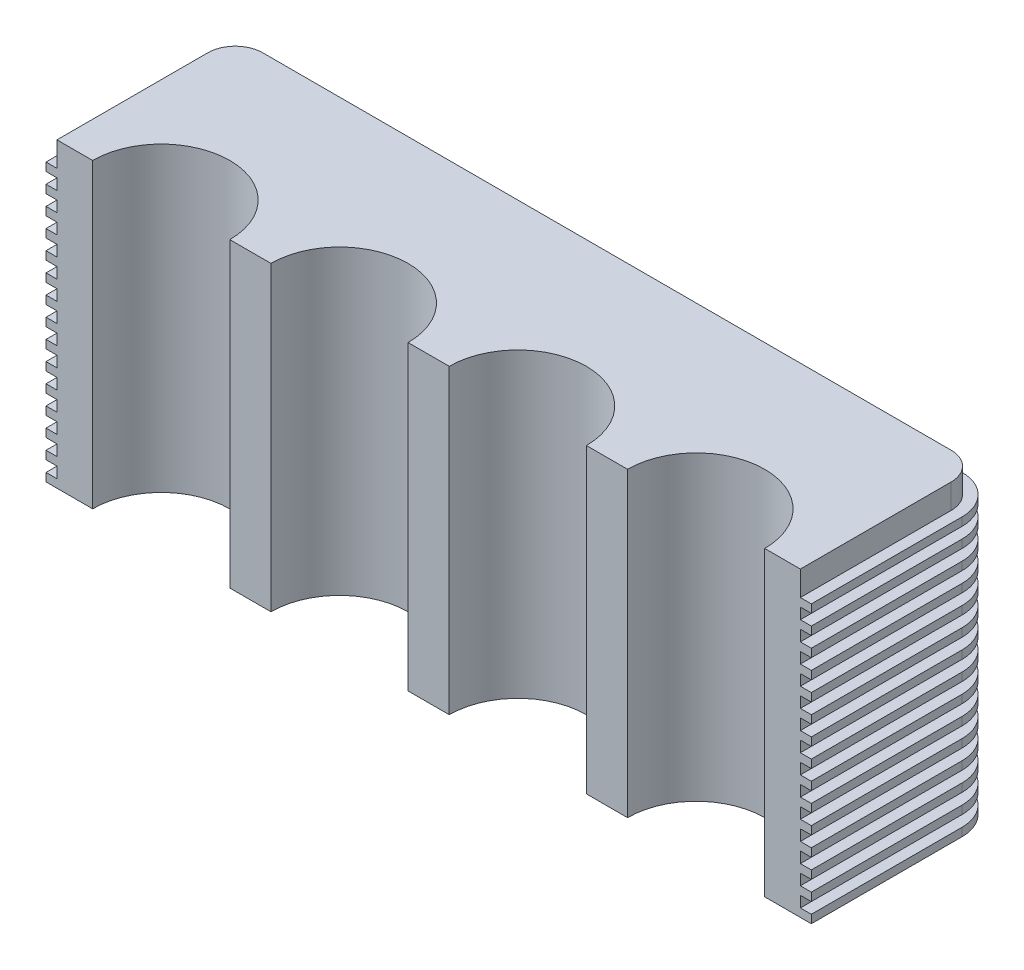
SolidWorks part; units mm, degrees
material "Plain Carbon Steel"
ref_plane "Front Plane" through (0, 0, 0) normal (0, 0, 1) x (1, 0, 0)
ref_plane "Top Plane" through (0, 0, 0) normal (0, 1, 0) x (1, 0, 0)
ref_plane "Right Plane" through (0, 0, 0) normal (1, 0, 0) x (0, 0, -1)
sketch "Block Profile Sketch" plane through (0, 0, 0) normal (0, 1, 0) x (1, 0, 0)
  line L0 (135.5, 0) -> (135.5, 65) construction
  line L1 (0, 0) -> (13, 0)
  line L2 (0, 0) -> (0, 55)
  line L3 (10, 65) -> (261, 65)
  line L4 (271, 0) -> (271, 55)
  line L5 (258, 0) -> (271, 0)
  line L6 (193, 0) -> (208, 0)
  line L7 (63, 0) -> (78, 0)
  line L8 (128, 0) -> (143, 0)
  arc A0 (261, 65) -> (271, 55) centre (261, 55) cw
  arc A1 (0, 55) -> (10, 65) centre (10, 55) cw
  arc A2 (258, 0) -> (208, 0) centre (233, 0) ccw
  arc A3 (193, 0) -> (143, 0) centre (168, 0) ccw
  arc A4 (13, 0) -> (63, 0) centre (38, 0) cw
  arc A5 (78, 0) -> (128, 0) centre (103, 0) cw
  dimension "D1" = 10
  dimension "D4" = 25
  dimension "D7" = 25
  dimension "D2" = 271
  dimension "D3" = 65
  dimension "D5" = 13
  dimension "D6" = 15
extrude "Upper Block Body" add sketch "Block Profile Sketch" along normal blind 110
sketch "End Serration Sketch" plane through (0, 0, 0) normal (0, 1, 0) x (1, 0, 0)
  line L0 (275, 0) -> (275, 55)
  line L1 (261, 69) -> (10, 69)
  line L2 (-4, 55) -> (-4, 0)
  line L3 (271, 0) -> (275, 0)
  line L4 (0, 0) -> (-4, 0)
  line L8 (0, 55) -> (0, 0)
  line L9 (0, 0) -> (13, 0)
  line L10 (63, 0) -> (78, 0)
  line L11 (128, 0) -> (143, 0)
  line L12 (193, 0) -> (208, 0)
  line L13 (258, 0) -> (271, 0)
  line L14 (271, 0) -> (271, 55)
  line L15 (261, 65) -> (10, 65)
  line L16 (0, 55) -> (0, 0)
  line L22 (271, 0) -> (271, 55)
  line L23 (261, 65) -> (10, 65)
  arc A0 (275, 55) -> (261, 69) centre (261, 55) ccw
  arc A1 (10, 69) -> (-4, 55) centre (10, 55) ccw
  arc A6 (63, 0) -> (13, 0) centre (38, 0) ccw
  arc A7 (128, 0) -> (78, 0) centre (103, 0) ccw
  arc A8 (193, 0) -> (143, 0) centre (168, 0) ccw
  arc A9 (258, 0) -> (208, 0) centre (233, 0) ccw
  arc A10 (271, 55) -> (261, 65) centre (261, 55) ccw
  arc A11 (10, 65) -> (0, 55) centre (10, 55) ccw
  arc A16 (271, 55) -> (261, 65) centre (261, 55) ccw
  arc A17 (10, 65) -> (0, 55) centre (10, 55) ccw
  dimension "D1" = 0
  dimension "D2" = 4
extrude "End Serration Rib" add sketch "End Serration Sketch" along normal blind 3
pattern_linear "Serration Rib Pattern 15x7mm" count 15 spacing 7 along (0, 1, 0) of "End Serration Rib"
